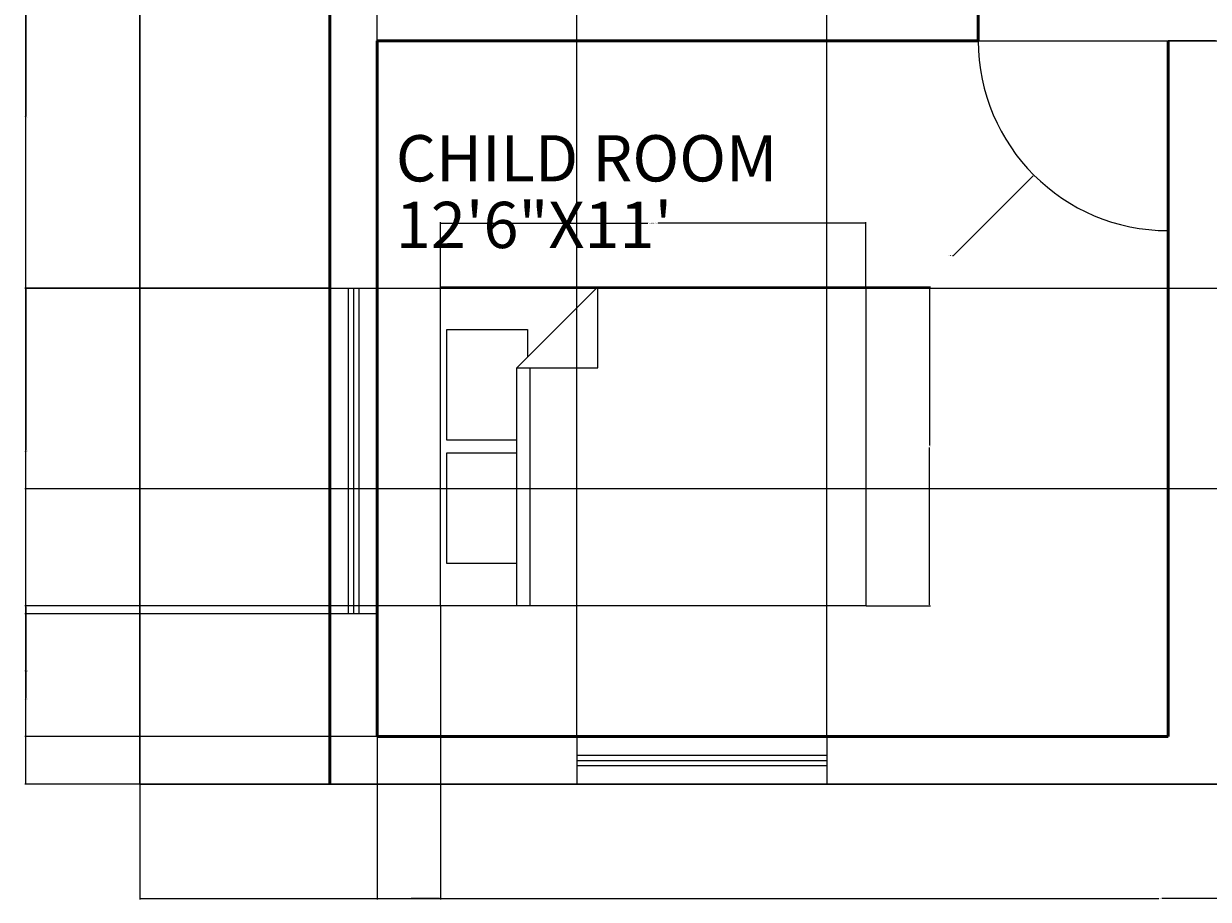
# Model space of a CAD drawing. Units: feet. Extents: x 2387 to 2818, y 1569 to 2046.
# Tile 1 of 4: x 2387 to 2611, y 1569 to 1735. Entities that reach past the tile are written whole.
import ezdxf

# ---------------------------------------------------------------- set-up
doc = ezdxf.new("R2010")
doc.units = ezdxf.units.FT
for name, color, linetype, lineweight in [('A-ANNO-DIMS', 2, 'Continuous', 18), ('A-AREA-IDEN', 7, 'Continuous', 18), ('A-DOOR', 3, 'Continuous', 25), ('A-FLOR-BALC', 7, 'Continuous', 30), ('A-FURN', 8, 'Continuous', 18), ('A-GLAZ', 4, 'Continuous', 18), ('A-WALL', 7, 'Continuous', 50)]:
    doc.layers.add(name, color=color, linetype=linetype, lineweight=lineweight)
doc.styles.get("Standard").update_dxf_attribs({"font": 'arial.ttf'})
doc.dimstyles.get("Standard").update_dxf_attribs({"dimtxt": 0.18, "dimasz": 0.18, "dimexe": 0.18, "dimexo": 0.0625, "dimgap": 0.09, "dimtad": 0, "dimtih": 1, "dimtoh": 1, "dimdec": 4, "dimzin": 0, "dimdsep": 46, "dimtxsty": 'Standard', "dimcen": 0.09, "dimadec": 0, "dimazin": 0, "dimtfac": 1, "dimtdec": 4, "dimtofl": 0, "dimtmove": 0, "dimatfit": 3, "dimfxl": 1, "dimtolj": 1, "dimtzin": 0, "dimarcsym": 0})

# ---------------------------------------------------------------- blocks, each defined once
blk = doc.blocks.new('Bed - Queen')
for p, q in [((0, -80.00003), (0, 0)), ((0, 0), (59.99999, 0)), ((59.99999, 0), (59.99999, -80.00003)), ((7.99999, -1.2), (28.79998, -1.2)), ((7.99999, -14.4), (7.99999, -1.2)), ((28.79998, -1.2), (28.79998, -14.4)), ((31.19999, -1.2), (51.99999, -1.2)), ((31.19999, -14.4), (31.19999, -1.2)), ((51.99999, -1.2), (51.99999, -16.4)), ((0, -14.4), (44.8, -14.4)), ((59.99999, -29.6), (44.8, -14.4)), ((44.8, -14.4), (44.8, -29.6)), ((44.8, -16.8), (0, -16.8)), ((51.99999, -16.4), (46.79936, -16.4)), ((44.8, -29.6), (59.99999, -29.6)), ((59.99999, -80.00003), (0, -80.00003))]:
    blk.add_line(p, q)
blk = doc.blocks.new('*D9')
at = {"layer": 'A-ANNO-DIMS', "color": 0, "lineweight": -2, "transparency": 16777216}
for p, q in [((2465.71, 1685.2), (2465.71, 1697.42)), ((2465.89, 1697.24), (2505.07, 1697.24)), ((2546.21, 1697.24), (2507.03, 1697.24)), ((2546.39, 1685.2), (2546.39, 1697.42))]:
    blk.add_line(p, q, dxfattribs=at)
at = {"layer": 'A-ANNO-DIMS', "color": 0, "transparency": 16777216}
for points in [[(2465.89, 1697.27), (2465.89, 1697.21), (2465.71, 1697.24)], [(2546.21, 1697.27), (2546.21, 1697.21), (2546.39, 1697.24)]]:
    blk.add_solid(points, dxfattribs=at)
at = {"layer": 'Defpoints', "color": 0, "transparency": 16777216}
for p in [(2465.71, 1697.24), (2465.71, 1685.14), (2546.39, 1685.14)]:
    blk.add_point(p, dxfattribs=at)
at = {"layer": 'A-ANNO-DIMS', "color": 0, "transparency": 16777216, "insert": (2506.05, 1697.24), "char_height": 0.18, "attachment_point": 5}
blk.add_mtext('\\A1;QUEEN BED 81', dxfattribs=at)
blk = doc.blocks.new('*D10')
at = {"layer": 'A-ANNO-DIMS', "color": 0, "lineweight": -2, "transparency": 16777216}
for p, q in [((2546.45, 1685.14), (2558.67, 1685.14)), ((2558.49, 1684.96), (2558.49, 1655.07)), ((2558.49, 1624.81), (2558.49, 1654.7)), ((2546.45, 1624.63), (2558.67, 1624.63))]:
    blk.add_line(p, q, dxfattribs=at)
at = {"layer": 'A-ANNO-DIMS', "color": 0, "transparency": 16777216}
for points in [[(2558.46, 1684.96), (2558.52, 1684.96), (2558.49, 1685.14)], [(2558.46, 1624.81), (2558.52, 1624.81), (2558.49, 1624.63)]]:
    blk.add_solid(points, dxfattribs=at)
at = {"layer": 'Defpoints', "color": 0, "transparency": 16777216}
for p in [(2546.39, 1685.14), (2558.49, 1685.14), (2546.39, 1624.63)]:
    blk.add_point(p, dxfattribs=at)
at = {"layer": 'A-ANNO-DIMS', "color": 0, "transparency": 16777216, "insert": (2558.49, 1654.89), "char_height": 0.18, "attachment_point": 5}
blk.add_mtext('\\A1;61', dxfattribs=at)
blk = doc.blocks.new('*D27')
at = {"layer": 'A-ANNO-DIMS', "color": 0, "lineweight": -2, "transparency": 16777216}
for p, q in [((2408.74, 1590.76), (2408.74, 1568.96)), ((2795.74, 1590.76), (2795.74, 1568.96)), ((2408.92, 1569.14), (2601.95, 1569.14)), ((2795.56, 1569.14), (2602.52, 1569.14))]:
    blk.add_line(p, q, dxfattribs=at)
at = {"layer": 'A-ANNO-DIMS', "color": 0, "transparency": 16777216}
for points in [[(2408.92, 1569.17), (2408.92, 1569.11), (2408.74, 1569.14)], [(2795.56, 1569.17), (2795.56, 1569.11), (2795.74, 1569.14)]]:
    blk.add_solid(points, dxfattribs=at)
at = {"layer": 'Defpoints', "color": 0, "transparency": 16777216}
for p in [(2408.74, 1590.82), (2795.74, 1590.82), (2795.74, 1569.14)]:
    blk.add_point(p, dxfattribs=at)
at = {"layer": 'A-ANNO-DIMS', "color": 0, "transparency": 16777216, "insert": (2602.24, 1569.14), "char_height": 0.18, "attachment_point": 5}
blk.add_mtext('\\A1;387', dxfattribs=at)
blk = doc.blocks.new('*D28')
at = {"layer": 'A-ANNO-DIMS', "color": 0, "lineweight": -2, "transparency": 16777216}
for p, q in [((2408.67, 2023.82), (2386.88, 2023.82)), ((2387.06, 2023.64), (2387.06, 1807.51)), ((2387.06, 1591), (2387.06, 1807.14)), ((2408.67, 1590.82), (2386.88, 1590.82))]:
    blk.add_line(p, q, dxfattribs=at)
at = {"layer": 'A-ANNO-DIMS', "color": 0, "transparency": 16777216}
for points in [[(2387.03, 2023.64), (2387.09, 2023.64), (2387.06, 2023.82)], [(2387.03, 1591), (2387.09, 1591), (2387.06, 1590.82)]]:
    blk.add_solid(points, dxfattribs=at)
at = {"layer": 'Defpoints', "color": 0, "transparency": 16777216}
for p in [(2387.06, 2023.82), (2408.74, 2023.82), (2408.74, 1590.82)]:
    blk.add_point(p, dxfattribs=at)
at = {"layer": 'A-ANNO-DIMS', "color": 0, "transparency": 16777216, "insert": (2387.06, 1807.32), "char_height": 0.18, "attachment_point": 5}
blk.add_mtext('\\A1;433', dxfattribs=at)
blk = doc.blocks.new('*D37')
at = {"layer": 'A-ANNO-DIMS', "color": 0, "lineweight": -2, "transparency": 16777216}
for p, q in [((2491.59, 1599.89), (2491.59, 2045.68)), ((2491.77, 2045.5), (2514.91, 2045.5)), ((2538.86, 2045.5), (2515.71, 2045.5)), ((2539.04, 1599.89), (2539.04, 2045.68))]:
    blk.add_line(p, q, dxfattribs=at)
at = {"layer": 'A-ANNO-DIMS', "color": 0, "transparency": 16777216}
for points in [[(2491.77, 2045.53), (2491.77, 2045.47), (2491.59, 2045.5)], [(2538.86, 2045.53), (2538.86, 2045.47), (2539.04, 2045.5)]]:
    blk.add_solid(points, dxfattribs=at)
at = {"layer": 'Defpoints', "color": 0, "transparency": 16777216}
for p in [(2539.04, 2045.5), (2491.59, 1599.82), (2539.04, 1599.82)]:
    blk.add_point(p, dxfattribs=at)
at = {"layer": 'A-ANNO-DIMS', "color": 0, "transparency": 16777216, "insert": (2515.31, 2045.5), "char_height": 0.18, "attachment_point": 5}
blk.add_mtext('\\A1;47.45', dxfattribs=at)
blk = doc.blocks.new('*D38')
at = {"layer": 'A-ANNO-DIMS', "color": 0, "lineweight": -2, "transparency": 16777216}
for p, q in [((2453.74, 1599.89), (2453.74, 2045.68)), ((2453.92, 2045.5), (2472.27, 2045.5)), ((2491.41, 2045.5), (2473.06, 2045.5)), ((2491.59, 1599.89), (2491.59, 2045.68))]:
    blk.add_line(p, q, dxfattribs=at)
at = {"layer": 'A-ANNO-DIMS', "color": 0, "transparency": 16777216}
for points in [[(2453.92, 2045.53), (2453.92, 2045.47), (2453.74, 2045.5)], [(2491.41, 2045.53), (2491.41, 2045.47), (2491.59, 2045.5)]]:
    blk.add_solid(points, dxfattribs=at)
at = {"layer": 'Defpoints', "color": 0, "transparency": 16777216}
for p in [(2491.59, 2045.5), (2453.74, 1599.82), (2491.59, 1599.82)]:
    blk.add_point(p, dxfattribs=at)
at = {"layer": 'A-ANNO-DIMS', "color": 0, "transparency": 16777216, "insert": (2472.66, 2045.5), "char_height": 0.18, "attachment_point": 5}
blk.add_mtext('\\A1;37.85', dxfattribs=at)
blk = doc.blocks.new('*D39')
at = {"layer": 'A-ANNO-DIMS', "color": 0, "lineweight": -2, "transparency": 16777216}
for p, q in [((2444.67, 1623.09), (2386.88, 1623.09)), ((2387.06, 1622.91), (2387.06, 1607.14)), ((2387.06, 1591), (2387.06, 1606.78)), ((2444.67, 1590.82), (2386.88, 1590.82))]:
    blk.add_line(p, q, dxfattribs=at)
at = {"layer": 'A-ANNO-DIMS', "color": 0, "transparency": 16777216}
for points in [[(2387.03, 1622.91), (2387.09, 1622.91), (2387.06, 1623.09)], [(2387.03, 1591), (2387.09, 1591), (2387.06, 1590.82)]]:
    blk.add_solid(points, dxfattribs=at)
at = {"layer": 'Defpoints', "color": 0, "transparency": 16777216}
for p in [(2387.06, 1623.09), (2444.74, 1623.09), (2444.74, 1590.82)]:
    blk.add_point(p, dxfattribs=at)
at = {"layer": 'A-ANNO-DIMS', "color": 0, "transparency": 16777216, "insert": (2387.06, 1606.96), "char_height": 0.18, "attachment_point": 5}
blk.add_mtext('\\A1;32.266', dxfattribs=at)
blk = doc.blocks.new('*D40')
at = {"layer": 'A-ANNO-DIMS', "color": 0, "lineweight": -2, "transparency": 16777216}
for p, q in [((2444.67, 1684.88), (2386.88, 1684.88)), ((2387.06, 1684.7), (2387.06, 1654.17)), ((2387.06, 1623.27), (2387.06, 1653.8)), ((2444.67, 1623.09), (2386.88, 1623.09))]:
    blk.add_line(p, q, dxfattribs=at)
at = {"layer": 'A-ANNO-DIMS', "color": 0, "transparency": 16777216}
for points in [[(2387.03, 1684.7), (2387.09, 1684.7), (2387.06, 1684.88)], [(2387.03, 1623.27), (2387.09, 1623.27), (2387.06, 1623.09)]]:
    blk.add_solid(points, dxfattribs=at)
at = {"layer": 'Defpoints', "color": 0, "transparency": 16777216}
for p in [(2387.06, 1684.88), (2444.74, 1684.88), (2444.74, 1623.09)]:
    blk.add_point(p, dxfattribs=at)
at = {"layer": 'A-ANNO-DIMS', "color": 0, "transparency": 16777216, "insert": (2387.06, 1653.99), "char_height": 0.18, "attachment_point": 5}
blk.add_mtext('\\A1;61.79', dxfattribs=at)
blk = doc.blocks.new('*D41')
at = {"layer": 'A-ANNO-DIMS', "color": 0, "lineweight": -2, "transparency": 16777216}
for p, q in [((2444.67, 1749.91), (2386.88, 1749.91)), ((2387.06, 1749.73), (2387.06, 1717.58)), ((2387.06, 1685.06), (2387.06, 1717.22)), ((2444.67, 1684.88), (2386.88, 1684.88))]:
    blk.add_line(p, q, dxfattribs=at)
at = {"layer": 'A-ANNO-DIMS', "color": 0, "transparency": 16777216}
for points in [[(2387.03, 1749.73), (2387.09, 1749.73), (2387.06, 1749.91)], [(2387.03, 1685.06), (2387.09, 1685.06), (2387.06, 1684.88)]]:
    blk.add_solid(points, dxfattribs=at)
at = {"layer": 'Defpoints', "color": 0, "transparency": 16777216}
for p in [(2387.06, 1749.91), (2444.74, 1749.91), (2444.74, 1684.88)]:
    blk.add_point(p, dxfattribs=at)
at = {"layer": 'A-ANNO-DIMS', "color": 0, "transparency": 16777216, "insert": (2387.06, 1717.4), "char_height": 0.18, "attachment_point": 5}
blk.add_mtext('\\A1;65.03', dxfattribs=at)
blk = doc.blocks.new('*D59')
at = {"layer": 'A-ANNO-DIMS', "color": 0, "lineweight": -2, "transparency": 16777216}
for p, q in [((2666.67, 1684.82), (2386.88, 1684.82)), ((2387.06, 1684.64), (2387.06, 1666.01)), ((2387.06, 1647), (2387.06, 1665.64)), ((2666.67, 1646.82), (2386.88, 1646.82))]:
    blk.add_line(p, q, dxfattribs=at)
at = {"layer": 'A-ANNO-DIMS', "color": 0, "transparency": 16777216}
for points in [[(2387.03, 1684.64), (2387.09, 1684.64), (2387.06, 1684.82)], [(2387.03, 1647), (2387.09, 1647), (2387.06, 1646.82)]]:
    blk.add_solid(points, dxfattribs=at)
at = {"layer": 'Defpoints', "color": 0, "transparency": 16777216}
for p in [(2666.74, 1684.82), (2387.06, 1646.82), (2666.74, 1646.82)]:
    blk.add_point(p, dxfattribs=at)
at = {"layer": 'A-ANNO-DIMS', "color": 0, "transparency": 16777216, "insert": (2387.06, 1665.82), "char_height": 0.18, "attachment_point": 5}
blk.add_mtext('\\A1;38', dxfattribs=at)
blk = doc.blocks.new('*D63')
at = {"layer": 'A-ANNO-DIMS', "color": 0, "lineweight": -2, "transparency": 16777216}
for p, q in [((2567.8, 1774.36), (2817.6, 1774.36)), ((2817.42, 1774.18), (2817.42, 1753.27)), ((2817.42, 1732), (2817.42, 1752.91)), ((2567.8, 1731.82), (2817.6, 1731.82))]:
    blk.add_line(p, q, dxfattribs=at)
at = {"layer": 'A-ANNO-DIMS', "color": 0, "transparency": 16777216}
for points in [[(2817.39, 1774.18), (2817.45, 1774.18), (2817.42, 1774.36)], [(2817.39, 1732), (2817.45, 1732), (2817.42, 1731.82)]]:
    blk.add_solid(points, dxfattribs=at)
at = {"layer": 'Defpoints', "color": 0, "transparency": 16777216}
for p in [(2567.74, 1774.36), (2817.42, 1774.36), (2567.74, 1731.82)]:
    blk.add_point(p, dxfattribs=at)
at = {"layer": 'A-ANNO-DIMS', "color": 0, "transparency": 16777216, "insert": (2817.42, 1753.09), "char_height": 0.18, "attachment_point": 5}
blk.add_mtext('\\A1;42.53', dxfattribs=at)
blk = doc.blocks.new('*D67')
at = {"layer": 'A-ANNO-DIMS', "color": 0, "lineweight": -2, "transparency": 16777216}
for p, q in [((2465.65, 1624.63), (2386.88, 1624.63)), ((2387.06, 1624.45), (2387.06, 1612.41)), ((2387.06, 1600), (2387.06, 1612.05)), ((2453.67, 1599.82), (2386.88, 1599.82))]:
    blk.add_line(p, q, dxfattribs=at)
at = {"layer": 'A-ANNO-DIMS', "color": 0, "transparency": 16777216}
for points in [[(2387.03, 1624.45), (2387.09, 1624.45), (2387.06, 1624.63)], [(2387.03, 1600), (2387.09, 1600), (2387.06, 1599.82)]]:
    blk.add_solid(points, dxfattribs=at)
at = {"layer": 'Defpoints', "color": 0, "transparency": 16777216}
for p in [(2465.71, 1624.63), (2387.06, 1599.82), (2453.74, 1599.82)]:
    blk.add_point(p, dxfattribs=at)
at = {"layer": 'A-ANNO-DIMS', "color": 0, "transparency": 16777216, "insert": (2387.06, 1612.23), "char_height": 0.18, "attachment_point": 5}
blk.add_mtext('\\A1;24.805', dxfattribs=at)
blk = doc.blocks.new('*D68')
at = {"layer": 'A-ANNO-DIMS', "color": 0, "lineweight": -2, "transparency": 16777216}
for p, q in [((2465.71, 1624.57), (2465.71, 1568.96)), ((2453.74, 1599.76), (2453.74, 1568.96)), ((2453.92, 1569.14), (2459.27, 1569.14)), ((2465.53, 1569.14), (2460.18, 1569.14))]:
    blk.add_line(p, q, dxfattribs=at)
at = {"layer": 'A-ANNO-DIMS', "color": 0, "transparency": 16777216}
for points in [[(2453.92, 1569.17), (2453.92, 1569.11), (2453.74, 1569.14)], [(2465.53, 1569.17), (2465.53, 1569.11), (2465.71, 1569.14)]]:
    blk.add_solid(points, dxfattribs=at)
at = {"layer": 'Defpoints', "color": 0, "transparency": 16777216}
for p in [(2465.71, 1624.63), (2453.74, 1599.82), (2453.74, 1569.14)]:
    blk.add_point(p, dxfattribs=at)
at = {"layer": 'A-ANNO-DIMS', "color": 0, "transparency": 16777216, "insert": (2459.72, 1569.14), "char_height": 0.18, "attachment_point": 5}
blk.add_mtext('\\A1;11.972', dxfattribs=at)
blk = doc.blocks.new('*D72')
at = {"layer": 'A-ANNO-DIMS', "color": 0, "lineweight": -2, "transparency": 16777216}
for p, q in [((2603.65, 1731.82), (2603.83, 1731.82)), ((2603.74, 1731.73), (2603.74, 1731.91)), ((2563.01, 1691.1), (2578.15, 1706.24)), ((2562.83, 1691.1), (2563.01, 1691.1))]:
    blk.add_line(p, q, dxfattribs=at)
at = {"layer": 'A-ANNO-DIMS', "color": 0, "transparency": 16777216}
blk.add_solid([(2578.13, 1706.26), (2578.17, 1706.22), (2578.28, 1706.37)], dxfattribs=at)
at = {"layer": 'Defpoints', "color": 0, "transparency": 16777216}
for p in [(2603.74, 1731.82), (2578.28, 1706.37)]:
    blk.add_point(p, dxfattribs=at)
at = {"layer": 'A-ANNO-DIMS', "color": 0, "transparency": 16777216, "insert": (2562.33, 1691.1), "char_height": 0.18, "attachment_point": 5}
blk.add_mtext('\\A1;2X R36', dxfattribs=at)

msp = doc.modelspace()

# ---------------------------------------------------------------- linework, layer by layer
at = {"layer": 'A-DOOR'}
for p, q in [((2612.736, 1731.8244), (2603.736, 1731.8244)), ((2603.736, 1731.8244), (2603.736, 1697.2244))]:
    msp.add_line(p, q, dxfattribs=at)
msp.add_arc((2603.736, 1731.8244), 36, 180, 270, dxfattribs=at)
at = {"layer": 'A-FLOR-BALC'}
for p, q in [((2408.736, 2023.8244), (2408.736, 1590.8244)), ((2408.736, 1590.8244), (2795.736, 1590.8244))]:
    msp.add_line(p, q, dxfattribs=at)
at = {"layer": 'A-GLAZ'}
for p, q in [((2444.736, 1684.8801), (2453.736, 1684.8801)), ((2448.236, 1684.8801), (2448.236, 1623.0908)), ((2449.236, 1684.8801), (2449.236, 1623.0908)), ((2450.236, 1684.8801), (2450.236, 1623.0908)), ((2453.736, 1623.0908), (2444.736, 1623.0908)), ((2491.5876, 1599.8244), (2491.5876, 1590.8244)), ((2539.0379, 1599.8244), (2539.0379, 1590.8244)), ((2491.5876, 1596.3244), (2539.0379, 1596.3244)), ((2491.5876, 1595.3244), (2539.0379, 1595.3244)), ((2491.5876, 1594.3244), (2539.0379, 1594.3244))]:
    msp.add_line(p, q, dxfattribs=at)
at = {"layer": 'A-WALL'}
for p, q in [((2444.736, 1590.8244), (2444.736, 1848.8244)), ((2567.736, 1731.8244), (2567.736, 1774.356)), ((2444.736, 1731.8244), (2444.736, 1590.8244)), ((2453.736, 1731.8244), (2567.736, 1731.8244)), ((2453.736, 1731.8244), (2453.736, 1599.8244)), ((2510.736, 1731.8244), (2558.736, 1731.8244)), ((2603.736, 1599.8244), (2603.736, 1731.8244)), ((2453.736, 1599.8244), (2603.736, 1599.8244))]:
    msp.add_line(p, q, dxfattribs=at)

# ---------------------------------------------------------------- block references
at = {"layer": 'A-FURN', "xscale": 1.008504331710163, "yscale": 1.008504331710163, "zscale": 1.008504331710163, "rotation": 90}
msp.add_blockref('Bed - Queen', (2465.708, 1624.6299), dxfattribs=at)

# ---------------------------------------------------------------- texts
at = {"layer": 'A-AREA-IDEN'}
for s, p in [('CHILD ROOM', (2457.2609, 1705.15)), ('12\'6"X11\'', (2457.2609, 1692.5076))]:
    msp.add_text(s, height=8.77438, dxfattribs=at).set_placement(p)

# ---------------------------------------------------------------- dimensions: what is measured, and where the dimension line sits
at = {"layer": 'A-ANNO-DIMS'}
for base, p1, p2, override, picture, middle in [((2491.5876, 2045.5044), (2453.736, 1599.8244), (2491.5876, 1599.8244), {"dimdec": 2, "dimlfac": 1, "dimrnd": 0, "dimzin": 0, "dimdsep": 46, "dimlunit": 2}, '*D38', (2472.6618, 2045.5044)), ((2539.0379, 2045.5044), (2491.5876, 1599.8244), (2539.0379, 1599.8244), {"dimdec": 2, "dimlfac": 1, "dimrnd": 0, "dimzin": 0, "dimdsep": 46, "dimlunit": 2}, '*D37', (2515.3128, 2045.5044)), ((2453.736, 1569.1444), (2465.708, 1624.6299), (2453.736, 1599.8244), {"dimdec": 3, "dimlfac": 1, "dimrnd": 0, "dimzin": 0, "dimdsep": 46, "dimlunit": 2}, '*D68', (2459.722, 1569.1444)), ((2795.736, 1569.1444), (2408.736, 1590.8244), (2795.736, 1590.8244), {"dimdec": 0, "dimlfac": 1, "dimrnd": 0, "dimzin": 0, "dimdsep": 46, "dimlunit": 2}, '*D27', (2602.236, 1569.1444))]:
    dim = msp.add_linear_dim(base=base, p1=p1, p2=p2, dimstyle='Standard', override=override, dxfattribs=at)
    dim.commit()
    dim.dimension.update_dxf_attribs({"geometry": picture, "text_midpoint": middle})
for base, p1, p2, override, picture, middle in [((2387.056, 2023.8244), (2408.736, 1590.8244), (2408.736, 2023.8244), {"dimdec": 0, "dimlfac": 1, "dimrnd": 0, "dimzin": 0, "dimdsep": 46, "dimlunit": 2}, '*D28', (2387.056, 1807.3244)), ((2817.416, 1774.356), (2567.736, 1731.8244), (2567.736, 1774.356), {"dimdec": 2, "dimlfac": 1, "dimrnd": 0, "dimzin": 0, "dimdsep": 46, "dimlunit": 2}, '*D63', (2817.416, 1753.0902)), ((2387.056, 1749.9143), (2444.736, 1684.8801), (2444.736, 1749.9143), {"dimdec": 2, "dimlfac": 1, "dimrnd": 0, "dimzin": 0, "dimdsep": 46, "dimlunit": 2}, '*D41', (2387.056, 1717.3972)), ((2558.4905, 1685.1401), (2546.3884, 1624.6299), (2546.3884, 1685.1401), {"dimdec": 0, "dimlfac": 1, "dimrnd": 0, "dimzin": 0, "dimdsep": 46, "dimlunit": 2}, '*D10', (2558.4905, 1654.885)), ((2387.056, 1684.8801), (2444.736, 1623.0908), (2444.736, 1684.8801), {"dimdec": 2, "dimlfac": 1, "dimrnd": 0, "dimzin": 0, "dimdsep": 46, "dimlunit": 2}, '*D40', (2387.056, 1653.9854)), ((2387.056, 1646.8244), (2666.736, 1684.8244), (2666.736, 1646.8244), {"dimdec": 0, "dimlfac": 1, "dimrnd": 0, "dimzin": 0, "dimdsep": 46, "dimlunit": 2}, '*D59', (2387.056, 1665.8244)), ((2387.05596, 1599.82441), (2465.70803, 1624.62988), (2453.73596, 1599.82441), {"dimdec": 3, "dimlfac": 1, "dimrnd": 0, "dimzin": 0, "dimdsep": 46, "dimlunit": 2}, '*D67', (2387.05596, 1612.22714)), ((2387.056, 1623.0908), (2444.736, 1590.8244), (2444.736, 1623.0908), {"dimdec": 3, "dimlfac": 1, "dimrnd": 0, "dimzin": 0, "dimdsep": 46, "dimlunit": 2}, '*D39', (2387.056, 1606.9576))]:
    dim = msp.add_linear_dim(base=base, p1=p1, p2=p2, angle=90, dimstyle='Standard', override=override, dxfattribs=at)
    dim.commit()
    dim.dimension.update_dxf_attribs({"geometry": picture, "text_midpoint": middle})
dim = msp.add_radius_dim(center=(2603.736, 1731.8244), mpoint=(2578.2798, 1706.3688), text='2X <>', dimstyle='Standard', override={"dimdec": 0, "dimlfac": 1, "dimrnd": 0, "dimzin": 0, "dimdsep": 46, "dimlunit": 2}, dxfattribs=at)
dim.commit()
dim.dimension.update_dxf_attribs({"geometry": '*D72', "text_midpoint": (2562.3263, 1691.0955), "dimtype": 164})
dim = msp.add_linear_dim(base=(2465.708, 1697.2422), p1=(2546.3884, 1685.1401), p2=(2465.708, 1685.1401), angle=180, text='QUEEN BED <>', dimstyle='Standard', override={"dimdec": 0, "dimlfac": 1, "dimrnd": 0, "dimzin": 0, "dimdsep": 46, "dimlunit": 2}, dxfattribs=at)
dim.commit()
dim.dimension.update_dxf_attribs({"geometry": '*D9', "text_midpoint": (2506.0482, 1697.2422)})

doc.saveas('drawing.dxf')
